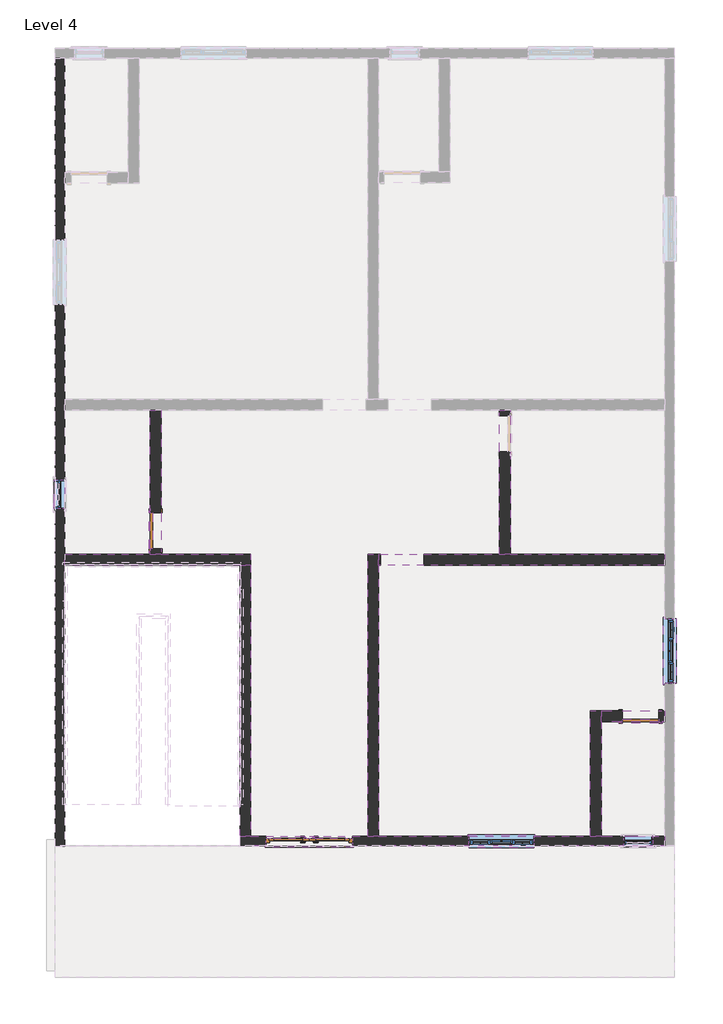
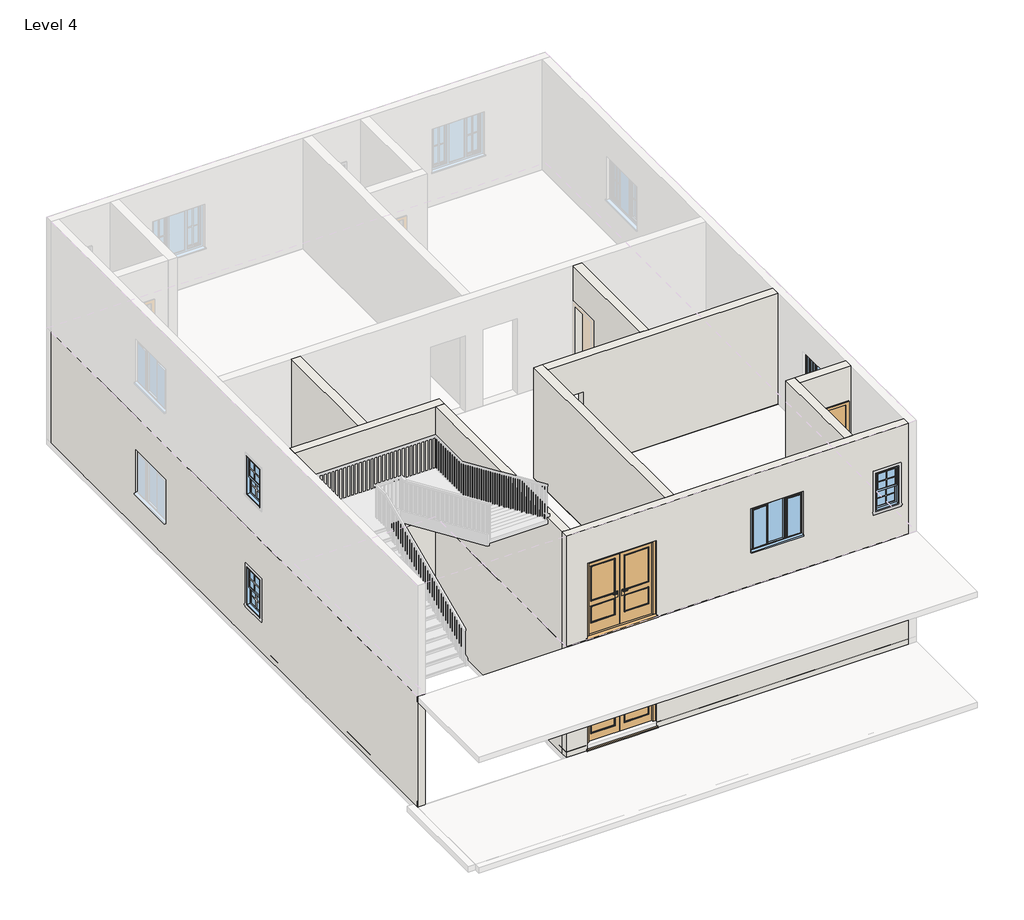
# One storey, part 1 of 5: 29 walls, 12 windows, 9 doors.
"""IFC4 building model written with IfcOpenShell, lengths in millimetres."""

from ifc_helpers import new_model, si_unit, frame, origin, place, context, project, spatial, polyline, outline, extrude, faceted_brep, transform, mapped, element, save
from components import doors_extdbl_2_1810x2110mm_9ab1935a, doors_extdbl_2_1810x2110mm_b7024f51, door_85036156, window_679d2811, windows_tpl_w_glazing_cross_bars_1360x1210mm_0306471f

model = new_model("IFC4")

# Units and contexts
model_context = context("Model", 3, world=origin())
ifc_project = project(units=[si_unit("LENGTHUNIT", "METRE", prefix="MILLI")], contexts=[model_context])

# Site, building, storey
site = spatial("IfcSite", under=ifc_project)
building = spatial("IfcBuilding", under=site)
storey = spatial("IfcBuildingStorey", under=building, Name="Level 4", Elevation=9144.0)

# Doors
placement = place(None, origin())
doors_extdbl_2_1810x2110mm_shape = doors_extdbl_2_1810x2110mm_9ab1935a(model_context)
doors_extdbl_2_1810x2110mm_2_shape = doors_extdbl_2_1810x2110mm_b7024f51(model_context)
element("IfcDoor", 1, ObjectType="Doors_ExtDbl_2 : 1810x2110mm", at=placement, inside=storey, context=model_context, shape_type="MappedRepresentation", body=[
    mapped(doors_extdbl_2_1810x2110mm_shape, transform((-2421.0852725, -7729.5064015, 9144.0), x_axis=(1.0, 0.0, 0.0), y_axis=(0.0, 1.0, 0.0), z_axis=(0.0, 0.0, 1.0))),
    mapped(doors_extdbl_2_1810x2110mm_2_shape, transform((-2421.0852725, -7729.5064015, 9144.0), x_axis=(1.0, 0.0, 0.0), y_axis=(0.0, 1.0, 0.0), z_axis=(0.0, 0.0, 1.0))),
])
element("IfcDoor", 2, ObjectType="Doors_ExtDbl_2 : 1810x2110mm", at=placement, inside=storey, context=model_context, shape_type="MappedRepresentation", body=[
    mapped(doors_extdbl_2_1810x2110mm_shape, transform((-2421.0852725, -7729.5064015, 9144.0), x_axis=(1.0, 0.0, 0.0), y_axis=(0.0, 1.0, 0.0), z_axis=(0.0, 0.0, 1.0))),
    mapped(doors_extdbl_2_1810x2110mm_2_shape, transform((-2421.0852725, -7729.5064015, 9144.0), x_axis=(1.0, 0.0, 0.0), y_axis=(0.0, 1.0, 0.0), z_axis=(0.0, 0.0, 1.0))),
])
element("IfcDoor", 3, ObjectType="Doors_ExtDbl_2 : 1810x2110mm", at=placement, inside=storey, context=model_context, shape_type="MappedRepresentation", body=[
    mapped(doors_extdbl_2_1810x2110mm_shape, transform((-2421.0852725, -7729.5064015, 12192.0), x_axis=(1.0, 0.0, 0.0), y_axis=(0.0, 1.0, 0.0), z_axis=(0.0, 0.0, 1.0))),
    mapped(doors_extdbl_2_1810x2110mm_2_shape, transform((-2421.0852725, -7729.5064015, 12192.0), x_axis=(1.0, 0.0, 0.0), y_axis=(0.0, 1.0, 0.0), z_axis=(0.0, 0.0, 1.0))),
])
door_shape = door_85036156(model_context)
element("IfcDoor", 4, ObjectType="Single-Flush : 30\" x 80\"", at=placement, inside=storey, context=model_context, shape_type="MappedRepresentation", body=[
    mapped(door_shape, transform((-5649.4415084, -1217.2217109, 9144.0), x_axis=(0.0, -1.0, 0.0), y_axis=(1.0, 0.0, 0.0), z_axis=(0.0, 0.0, 1.0))),
])
element("IfcDoor", 5, ObjectType="Single-Flush : 30\" x 80\"", at=placement, inside=storey, context=model_context, shape_type="MappedRepresentation", body=[
    mapped(door_shape, transform((4535.9584916, -5113.3064015, 9144.0), x_axis=(1.0, 0.0, 0.0), y_axis=(0.0, 1.0, 0.0), z_axis=(0.0, 0.0, 1.0))),
])
element("IfcDoor", 6, ObjectType="Single-Flush : 30\" x 80\"", at=placement, inside=storey, context=model_context, shape_type="MappedRepresentation", body=[
    mapped(door_shape, transform((-5649.4415084, -1217.2217109, 9144.0), x_axis=(0.0, -1.0, 0.0), y_axis=(1.0, 0.0, 0.0), z_axis=(0.0, 0.0, 1.0))),
])
element("IfcDoor", 7, ObjectType="Single-Flush : 30\" x 80\"", at=placement, inside=storey, context=model_context, shape_type="MappedRepresentation", body=[
    mapped(door_shape, transform((4535.9584916, -5113.3064015, 9144.0), x_axis=(1.0, 0.0, 0.0), y_axis=(0.0, 1.0, 0.0), z_axis=(0.0, 0.0, 1.0))),
])
element("IfcDoor", 8, ObjectType="Single-Flush : 30\" x 80\"", at=placement, inside=storey, context=model_context, shape_type="MappedRepresentation", body=[
    mapped(door_shape, transform((-5649.4415084, -1217.2217109, 12192.0), x_axis=(0.0, -1.0, 0.0), y_axis=(1.0, 0.0, 0.0), z_axis=(0.0, 0.0, 1.0))),
])
element("IfcDoor", 9, ObjectType="Single-Flush : 30\" x 80\"", at=placement, inside=storey, context=model_context, shape_type="MappedRepresentation", body=[
    mapped(door_shape, transform((4535.9584916, -5113.3064015, 12192.0), x_axis=(1.0, 0.0, 0.0), y_axis=(0.0, 1.0, 0.0), z_axis=(0.0, 0.0, 1.0))),
])

# Walls
element("IfcWall", 10, ObjectType="Generic - 4.5\"", at=placement, inside=storey, context=model_context, shape_type="SweptSolid", body=[
    extrude(outline(polyline([(-1598.2217109, 11176.0), (-1598.2217109, 9144.0), (-1712.5217109, 9144.0), (-1712.5217109, 12192.0), (1312.8935985, 12192.0), (1312.8935985, 9144.0), (-836.2217109, 9144.0), (-836.2217109, 11176.0), (-1598.2217109, 11176.0)])), frame((-5763.7415084, 0.0, 0.0), z_axis=(1.0, 0.0, 0.0), x_axis=(0.0, 1.0, 0.0)), (0.0, 0.0, 1.0), 228.6),
])
element("IfcWall", 11, ObjectType="Generic - 4.5\"", at=placement, inside=storey, context=model_context, shape_type="Brep", body=[
    faceted_brep([(-7554.4415084, -1941.1217109, 9144.0), (-3879.0290366, -1941.1217109, 9144.0), (-3650.4290366, -1941.1217109, 9144.0), (-3650.4290366, -1941.1217109, 12192.0), (-3879.0290366, -1941.1217109, 12192.0), (-7554.4415084, -1941.1217109, 12192.0), (-7554.4415084, -1712.5217109, 9144.0), (-7554.4415084, -1712.5217109, 12192.0), (-5763.7415084, -1712.5217109, 12192.0), (-5535.1415084, -1712.5217109, 12192.0), (-3650.4290366, -1712.5217109, 12192.0), (-3650.4290366, -1712.5217109, 9144.0), (-5535.1415084, -1712.5217109, 9144.0), (-5763.7415084, -1712.5217109, 9144.0)], [[[0, 1, 2, 3, 4, 5]], [[6, 7, 8, 9, 10, 11, 12, 13]], [[2, 1, 0, 6, 13, 12, 11]], [[5, 4, 3, 10, 9, 8, 7]], [[0, 5, 7, 6]], [[3, 2, 11, 10]]]),
])
element("IfcWall", 12, ObjectType="Generic - 4.5\"", at=placement, inside=storey, context=model_context, shape_type="SweptSolid", body=[
    extrude(outline(polyline([(-3879.0290366, -7627.9064015), (-3879.0290366, -1941.1217109), (-3650.4290366, -1941.1217109), (-3650.4290366, -7627.9064015), (-3879.0290366, -7627.9064015)])), frame((0.0, 0.0, 9144.0), z_axis=(0.0, 0.0, 1.0), x_axis=(1.0, 0.0, 0.0)), (0.0, 0.0, 1.0), 3048.0),
])
element("IfcWall", 13, ObjectType="Generic - 4.5\"", at=placement, inside=storey, context=model_context, shape_type="SweptSolid", body=[
    extrude(outline(polyline([(1312.8935985, 9144.0), (1198.5935985, 9144.0), (1198.5935985, 11176.0), (436.5935985, 11176.0), (436.5935985, 9144.0), (-1712.5217109, 9144.0), (-1712.5217109, 12192.0), (1312.8935985, 12192.0), (1312.8935985, 9144.0)])), frame((1576.8584916, 0.0, 0.0), z_axis=(1.0, 0.0, 0.0), x_axis=(0.0, 1.0, 0.0)), (0.0, 0.0, 1.0), 228.6),
])
element("IfcWall", 14, ObjectType="Generic - 4.5\"", at=placement, inside=storey, context=model_context, shape_type="Brep", body=[
    faceted_brep([(-963.1415084, -7627.9064015, 9144.0), (-963.1415084, -1941.1217109, 9144.0), (-963.1415084, -1712.5217109, 9144.0), (-963.1415084, -1712.5217109, 12192.0), (-963.1415084, -1941.1217109, 12192.0), (-963.1415084, -7627.9064015, 12192.0), (-1191.7415084, -7627.9064015, 9144.0), (-1191.7415084, -7627.9064015, 12192.0), (-1191.7415084, -1712.5217109, 12192.0), (-1191.7415084, -1712.5217109, 9144.0)], [[[0, 1, 2, 3, 4, 5]], [[6, 7, 8, 9]], [[2, 1, 0, 6, 9]], [[5, 4, 3, 8, 7]], [[0, 5, 7, 6]], [[3, 2, 9, 8]]]),
])
element("IfcWall", 15, ObjectType="Generic - 4.5\"", at=placement, inside=storey, context=model_context, shape_type="Brep", body=[
    faceted_brep([(-922.8415084, -1712.5217109, 11254.0), (-922.8415084, -1712.5217109, 9144.0), (-963.1415084, -1712.5217109, 9144.0), (-963.1415084, -1712.5217109, 12192.0), (1576.8584916, -1712.5217109, 12192.0), (1805.4584916, -1712.5217109, 12192.0), (5043.9584916, -1712.5217109, 12192.0), (5043.9584916, -1712.5217109, 9144.0), (1805.4584916, -1712.5217109, 9144.0), (1576.8584916, -1712.5217109, 9144.0), (-12.8415084, -1712.5217109, 9144.0), (-12.8415084, -1712.5217109, 11254.0), (-963.1415084, -1941.1217109, 9144.0), (-922.8415084, -1941.1217109, 9144.0), (-922.8415084, -1941.1217109, 11254.0), (-12.8415084, -1941.1217109, 11254.0), (-12.8415084, -1941.1217109, 9144.0), (5043.9584916, -1941.1217109, 9144.0), (5043.9584916, -1941.1217109, 12192.0), (-963.1415084, -1941.1217109, 12192.0)], [[[0, 1, 2, 3, 4, 5, 6, 7, 8, 9, 10, 11]], [[12, 13, 14, 15, 16, 17, 18, 19]], [[2, 1, 13, 12]], [[10, 9, 8, 7, 17, 16]], [[6, 5, 4, 3, 19, 18]], [[3, 2, 12, 19]], [[7, 6, 18, 17]], [[16, 15, 11, 10]], [[14, 13, 1, 0]], [[15, 14, 0, 11]]]),
])
element("IfcWall", 16, ObjectType="Generic - 4.5\"", at=placement, inside=storey, context=model_context, shape_type="Brep", body=[
    faceted_brep([(3710.4584916, -7627.9064015, 9144.0), (3710.4584916, -5227.6064015, 9144.0), (3710.4584916, -4999.0064015, 9144.0), (3710.4584916, -4999.0064015, 12192.0), (3710.4584916, -5227.6064015, 12192.0), (3710.4584916, -7627.9064015, 12192.0), (3481.8584916, -7627.9064015, 9144.0), (3481.8584916, -7627.9064015, 12192.0), (3481.8584916, -4999.0064015, 12192.0), (3481.8584916, -4999.0064015, 9144.0)], [[[0, 1, 2, 3, 4, 5]], [[6, 7, 8, 9]], [[2, 1, 0, 6, 9]], [[5, 4, 3, 8, 7]], [[0, 5, 7, 6]], [[3, 2, 9, 8]]]),
])
element("IfcWall", 17, ObjectType="Generic - 4.5\"", at=placement, inside=storey, context=model_context, shape_type="SweptSolid", body=[
    extrude(outline(polyline([(11176.0, 4916.9584916), (9144.0, 4916.9584916), (9144.0, 5043.9584916), (12192.0, 5043.9584916), (12192.0, 3710.4584916), (9144.0, 3710.4584916), (9144.0, 4154.9584916), (11176.0, 4154.9584916), (11176.0, 4916.9584916)])), frame((0.0, -5227.6064015, 0.0), z_axis=(0.0, 1.0, 0.0), x_axis=(0.0, 0.0, 1.0)), (0.0, 0.0, 1.0), 228.6),
])
element("IfcWall", 18, ObjectType="Generic - 4.5\"", at=placement, inside=storey, context=model_context, shape_type="SweptSolid", body=[
    extrude(outline(polyline([(-1598.2217109, 11176.0), (-1598.2217109, 9144.0), (-1712.5217109, 9144.0), (-1712.5217109, 12192.0), (1312.8935985, 12192.0), (1312.8935985, 9144.0), (-836.2217109, 9144.0), (-836.2217109, 11176.0), (-1598.2217109, 11176.0)])), frame((-5763.7415084, 0.0, 0.0), z_axis=(1.0, 0.0, 0.0), x_axis=(0.0, 1.0, 0.0)), (0.0, 0.0, 1.0), 228.6),
])
element("IfcWall", 19, ObjectType="Generic - 4.5\"", at=placement, inside=storey, context=model_context, shape_type="Brep", body=[
    faceted_brep([(-7554.4415084, -1941.1217109, 9144.0), (-3879.0290366, -1941.1217109, 9144.0), (-3879.0290366, -1941.1217109, 12192.0), (-7554.4415084, -1941.1217109, 12192.0), (-7554.4415084, -1712.5217109, 9144.0), (-7554.4415084, -1712.5217109, 12192.0), (-5763.7415084, -1712.5217109, 12192.0), (-5535.1415084, -1712.5217109, 12192.0), (-3879.0290366, -1712.5217109, 12192.0), (-3879.0290366, -1712.5217109, 9144.0), (-5535.1415084, -1712.5217109, 9144.0), (-5763.7415084, -1712.5217109, 9144.0)], [[[0, 1, 2, 3]], [[4, 5, 6, 7, 8, 9, 10, 11]], [[1, 0, 4, 11, 10, 9]], [[3, 2, 8, 7, 6, 5]], [[0, 3, 5, 4]], [[2, 1, 9, 8]]]),
])
element("IfcWall", 20, ObjectType="Generic - 4.5\"", at=placement, inside=storey, context=model_context, shape_type="SweptSolid", body=[
    extrude(outline(polyline([(-3879.0290366, -7627.9064015), (-3879.0290366, -1941.1217109), (-3650.4290366, -1941.1217109), (-3650.4290366, -7627.9064015), (-3879.0290366, -7627.9064015)])), frame((0.0, 0.0, 9144.0), z_axis=(0.0, 0.0, 1.0), x_axis=(1.0, 0.0, 0.0)), (0.0, 0.0, 1.0), 3048.0),
])
element("IfcWall", 21, ObjectType="Generic - 4.5\"", at=placement, inside=storey, context=model_context, shape_type="SweptSolid", body=[
    extrude(outline(polyline([(1312.8935985, 9144.0), (1198.5935985, 9144.0), (1198.5935985, 11176.0), (436.5935985, 11176.0), (436.5935985, 9144.0), (-1712.5217109, 9144.0), (-1712.5217109, 12192.0), (1312.8935985, 12192.0), (1312.8935985, 9144.0)])), frame((1576.8584916, 0.0, 0.0), z_axis=(1.0, 0.0, 0.0), x_axis=(0.0, 1.0, 0.0)), (0.0, 0.0, 1.0), 228.6),
])
element("IfcWall", 22, ObjectType="Generic - 4.5\"", at=placement, inside=storey, context=model_context, shape_type="SweptSolid", body=[
    extrude(outline(polyline([(-963.1415084, -1941.1217109), (-963.1415084, -7627.9064015), (-1191.7415084, -7627.9064015), (-1191.7415084, -1941.1217109), (-963.1415084, -1941.1217109)])), frame((0.0, 0.0, 9144.0), z_axis=(0.0, 0.0, 1.0), x_axis=(1.0, 0.0, 0.0)), (0.0, 0.0, 1.0), 3048.0),
])
element("IfcWall", 23, ObjectType="Generic - 4.5\"", at=placement, inside=storey, context=model_context, shape_type="Brep", body=[
    faceted_brep([(-922.8415084, -1712.5217109, 11254.0), (-922.8415084, -1712.5217109, 9144.0), (-963.1415084, -1712.5217109, 9144.0), (-963.1415084, -1712.5217109, 12192.0), (1576.8584916, -1712.5217109, 12192.0), (1805.4584916, -1712.5217109, 12192.0), (5043.9584916, -1712.5217109, 12192.0), (5043.9584916, -1712.5217109, 9144.0), (1805.4584916, -1712.5217109, 9144.0), (1576.8584916, -1712.5217109, 9144.0), (-12.8415084, -1712.5217109, 9144.0), (-12.8415084, -1712.5217109, 11254.0), (-963.1415084, -1941.1217109, 9144.0), (-922.8415084, -1941.1217109, 9144.0), (-922.8415084, -1941.1217109, 11254.0), (-12.8415084, -1941.1217109, 11254.0), (-12.8415084, -1941.1217109, 9144.0), (5043.9584916, -1941.1217109, 9144.0), (5043.9584916, -1941.1217109, 12192.0), (-963.1415084, -1941.1217109, 12192.0)], [[[0, 1, 2, 3, 4, 5, 6, 7, 8, 9, 10, 11]], [[12, 13, 14, 15, 16, 17, 18, 19]], [[2, 1, 13, 12]], [[10, 9, 8, 7, 17, 16]], [[6, 5, 4, 3, 19, 18]], [[7, 6, 18, 17]], [[16, 15, 11, 10]], [[14, 13, 1, 0]], [[15, 14, 0, 11]], [[3, 2, 12, 19]]]),
])
element("IfcWall", 24, ObjectType="Generic - 4.5\"", at=placement, inside=storey, context=model_context, shape_type="SweptSolid", body=[
    extrude(outline(polyline([(3710.4584916, -5227.6064015), (3710.4584916, -7627.9064015), (3481.8584916, -7627.9064015), (3481.8584916, -5227.6064015), (3710.4584916, -5227.6064015)])), frame((0.0, 0.0, 9144.0), z_axis=(0.0, 0.0, 1.0), x_axis=(1.0, 0.0, 0.0)), (0.0, 0.0, 1.0), 3048.0),
])
element("IfcWall", 25, ObjectType="Generic - 4.5\"", at=placement, inside=storey, context=model_context, shape_type="SweptSolid", body=[
    extrude(outline(polyline([(11176.0, 4916.9584916), (9144.0, 4916.9584916), (9144.0, 5043.9584916), (12192.0, 5043.9584916), (12192.0, 3710.4584916), (9144.0, 3710.4584916), (9144.0, 4154.9584916), (11176.0, 4154.9584916), (11176.0, 4916.9584916)])), frame((0.0, -5227.6064015, 0.0), z_axis=(0.0, 1.0, 0.0), x_axis=(0.0, 0.0, 1.0)), (0.0, 0.0, 1.0), 228.6),
])
element("IfcWall", 26, ObjectType="Generic - 4.5\"", at=placement, inside=storey, context=model_context, shape_type="SweptSolid", body=[
    extrude(outline(polyline([(-1598.2217109, 14224.0), (-1598.2217109, 12192.0), (-1712.5217109, 12192.0), (-1712.5217109, 15240.0), (1312.8935985, 15240.0), (1312.8935985, 12192.0), (-836.2217109, 12192.0), (-836.2217109, 14224.0), (-1598.2217109, 14224.0)])), frame((-5763.7415084, 0.0, 0.0), z_axis=(1.0, 0.0, 0.0), x_axis=(0.0, 1.0, 0.0)), (0.0, 0.0, 1.0), 228.6),
])
element("IfcWall", 27, ObjectType="Generic - 4.5\"", at=placement, inside=storey, context=model_context, shape_type="Brep", body=[
    faceted_brep([(-7554.4415084, -1941.1217109, 12192.0), (-3879.0290366, -1941.1217109, 12192.0), (-3650.4290366, -1941.1217109, 12192.0), (-3650.4290366, -1941.1217109, 15240.0), (-3879.0290366, -1941.1217109, 15240.0), (-7554.4415084, -1941.1217109, 15240.0), (-7554.4415084, -1712.5217109, 12192.0), (-7554.4415084, -1712.5217109, 15240.0), (-5763.7415084, -1712.5217109, 15240.0), (-5535.1415084, -1712.5217109, 15240.0), (-3650.4290366, -1712.5217109, 15240.0), (-3650.4290366, -1712.5217109, 12192.0), (-5535.1415084, -1712.5217109, 12192.0), (-5763.7415084, -1712.5217109, 12192.0)], [[[0, 1, 2, 3, 4, 5]], [[6, 7, 8, 9, 10, 11, 12, 13]], [[2, 1, 0, 6, 13, 12, 11]], [[5, 4, 3, 10, 9, 8, 7]], [[0, 5, 7, 6]], [[3, 2, 11, 10]]]),
])
element("IfcWall", 28, ObjectType="Generic - 4.5\"", at=placement, inside=storey, context=model_context, shape_type="SweptSolid", body=[
    extrude(outline(polyline([(-3879.0290366, -7627.9064015), (-3879.0290366, -1941.1217109), (-3650.4290366, -1941.1217109), (-3650.4290366, -7627.9064015), (-3879.0290366, -7627.9064015)])), frame((0.0, 0.0, 12192.0), z_axis=(0.0, 0.0, 1.0), x_axis=(1.0, 0.0, 0.0)), (0.0, 0.0, 1.0), 3048.0),
])
element("IfcWall", 29, ObjectType="Generic - 4.5\"", at=placement, inside=storey, context=model_context, shape_type="SweptSolid", body=[
    extrude(outline(polyline([(1312.8935985, 12192.0), (1198.5935985, 12192.0), (1198.5935985, 14224.0), (436.5935985, 14224.0), (436.5935985, 12192.0), (-1712.5217109, 12192.0), (-1712.5217109, 15240.0), (1312.8935985, 15240.0), (1312.8935985, 12192.0)])), frame((1576.8584916, 0.0, 0.0), z_axis=(1.0, 0.0, 0.0), x_axis=(0.0, 1.0, 0.0)), (0.0, 0.0, 1.0), 228.6),
])
element("IfcWall", 30, ObjectType="Generic - 4.5\"", at=placement, inside=storey, context=model_context, shape_type="Brep", body=[
    faceted_brep([(-963.1415084, -7627.9064015, 12192.0), (-963.1415084, -1941.1217109, 12192.0), (-963.1415084, -1712.5217109, 12192.0), (-963.1415084, -1712.5217109, 15240.0), (-963.1415084, -1941.1217109, 15240.0), (-963.1415084, -7627.9064015, 15240.0), (-1191.7415084, -7627.9064015, 12192.0), (-1191.7415084, -7627.9064015, 15240.0), (-1191.7415084, -1712.5217109, 15240.0), (-1191.7415084, -1712.5217109, 12192.0)], [[[0, 1, 2, 3, 4, 5]], [[6, 7, 8, 9]], [[2, 1, 0, 6, 9]], [[5, 4, 3, 8, 7]], [[0, 5, 7, 6]], [[3, 2, 9, 8]]]),
])
element("IfcWall", 31, ObjectType="Generic - 4.5\"", at=placement, inside=storey, context=model_context, shape_type="Brep", body=[
    faceted_brep([(-922.8415084, -1712.5217109, 14302.0), (-922.8415084, -1712.5217109, 12192.0), (-963.1415084, -1712.5217109, 12192.0), (-963.1415084, -1712.5217109, 15240.0), (1576.8584916, -1712.5217109, 15240.0), (1805.4584916, -1712.5217109, 15240.0), (5043.9584916, -1712.5217109, 15240.0), (5043.9584916, -1712.5217109, 12192.0), (1805.4584916, -1712.5217109, 12192.0), (1576.8584916, -1712.5217109, 12192.0), (-12.8415084, -1712.5217109, 12192.0), (-12.8415084, -1712.5217109, 14302.0), (-963.1415084, -1941.1217109, 12192.0), (-922.8415084, -1941.1217109, 12192.0), (-922.8415084, -1941.1217109, 14302.0), (-12.8415084, -1941.1217109, 14302.0), (-12.8415084, -1941.1217109, 12192.0), (5043.9584916, -1941.1217109, 12192.0), (5043.9584916, -1941.1217109, 15240.0), (-963.1415084, -1941.1217109, 15240.0)], [[[0, 1, 2, 3, 4, 5, 6, 7, 8, 9, 10, 11]], [[12, 13, 14, 15, 16, 17, 18, 19]], [[2, 1, 13, 12]], [[10, 9, 8, 7, 17, 16]], [[6, 5, 4, 3, 19, 18]], [[3, 2, 12, 19]], [[7, 6, 18, 17]], [[16, 15, 11, 10]], [[14, 13, 1, 0]], [[15, 14, 0, 11]]]),
])
element("IfcWall", 32, ObjectType="Generic - 4.5\"", at=placement, inside=storey, context=model_context, shape_type="Brep", body=[
    faceted_brep([(3710.4584916, -7627.9064015, 12192.0), (3710.4584916, -5227.6064015, 12192.0), (3710.4584916, -4999.0064015, 12192.0), (3710.4584916, -4999.0064015, 15240.0), (3710.4584916, -5227.6064015, 15240.0), (3710.4584916, -7627.9064015, 15240.0), (3481.8584916, -7627.9064015, 12192.0), (3481.8584916, -7627.9064015, 15240.0), (3481.8584916, -4999.0064015, 15240.0), (3481.8584916, -4999.0064015, 12192.0)], [[[0, 1, 2, 3, 4, 5]], [[6, 7, 8, 9]], [[2, 1, 0, 6, 9]], [[5, 4, 3, 8, 7]], [[0, 5, 7, 6]], [[3, 2, 9, 8]]]),
])
element("IfcWall", 33, ObjectType="Generic - 4.5\"", at=placement, inside=storey, context=model_context, shape_type="SweptSolid", body=[
    extrude(outline(polyline([(14224.0, 4916.9584916), (12192.0, 4916.9584916), (12192.0, 5043.9584916), (15240.0, 5043.9584916), (15240.0, 3710.4584916), (12192.0, 3710.4584916), (12192.0, 4154.9584916), (14224.0, 4154.9584916), (14224.0, 4916.9584916)])), frame((0.0, -5227.6064015, 0.0), z_axis=(0.0, 1.0, 0.0), x_axis=(0.0, 0.0, 1.0)), (0.0, 0.0, 1.0), 228.6),
])
element("IfcWall", 34, ObjectType="Generic - 9\"", at=placement, inside=storey, context=model_context, shape_type="Brep", body=[
    faceted_brep([(5043.9584916, -7627.9064015, 9144.0), (3710.4584916, -7627.9064015, 9144.0), (3481.8584916, -7627.9064015, 9144.0), (-963.1415084, -7627.9064015, 9144.0), (-1191.7415084, -7627.9064015, 9144.0), (-1516.0852725, -7627.9064015, 9144.0), (-1516.0852725, -7627.9064015, 11254.0), (-3326.0852725, -7627.9064015, 11254.0), (-3326.0852725, -7627.9064015, 9144.0), (-3650.4290366, -7627.9064015, 9144.0), (-3879.0290366, -7627.9064015, 9144.0), (-3879.0290366, -7627.9064015, 12192.0), (-3650.4290366, -7627.9064015, 12192.0), (-1191.7415084, -7627.9064015, 12192.0), (-963.1415084, -7627.9064015, 12192.0), (3481.8584916, -7627.9064015, 12192.0), (3710.4584916, -7627.9064015, 12192.0), (5043.9584916, -7627.9064015, 12192.0), (2294.9584916, -7627.9064015, 11268.4), (934.9584916, -7627.9064015, 11268.4), (934.9584916, -7627.9064015, 10058.4), (2294.9584916, -7627.9064015, 10058.4), (4789.9584916, -7627.9064015, 11125.2), (4180.3584916, -7627.9064015, 11125.2), (4180.3584916, -7627.9064015, 10058.4), (4789.9584916, -7627.9064015, 10058.4), (-1516.0852725, -7831.1064015, 11254.0), (-1516.0852725, -7831.1064015, 9144.0), (5043.9584916, -7831.1064015, 9144.0), (5043.9584916, -7831.1064015, 12192.0), (-3879.0290366, -7831.1064015, 12192.0), (-3879.0290366, -7831.1064015, 9144.0), (-3326.0852725, -7831.1064015, 9144.0), (-3326.0852725, -7831.1064015, 11254.0), (2294.9584916, -7831.1064015, 11268.4), (2294.9584916, -7831.1064015, 10058.4), (934.9584916, -7831.1064015, 10058.4), (934.9584916, -7831.1064015, 11268.4), (4789.9584916, -7831.1064015, 11125.2), (4789.9584916, -7831.1064015, 10058.4), (4180.3584916, -7831.1064015, 10058.4), (4180.3584916, -7831.1064015, 11125.2)], [[[0, 1, 2, 3, 4, 5, 6, 7, 8, 9, 10, 11, 12, 13, 14, 15, 16, 17], [18, 19, 20, 21], [22, 23, 24, 25]], [[26, 27, 28, 29, 30, 31, 32, 33], [34, 35, 36, 37], [38, 39, 40, 41]], [[32, 31, 10, 9, 8]], [[28, 27, 5, 4, 3, 2, 1, 0]], [[17, 16, 15, 14, 13, 12, 11, 30, 29]], [[11, 10, 31, 30]], [[35, 34, 18, 21]], [[36, 35, 21, 20]], [[37, 36, 20, 19]], [[34, 37, 19, 18]], [[39, 38, 22, 25]], [[40, 39, 25, 24]], [[41, 40, 24, 23]], [[38, 41, 23, 22]], [[8, 7, 33, 32]], [[6, 5, 27, 26]], [[7, 6, 26, 33]], [[0, 17, 29, 28]]]),
])
element("IfcWall", 35, ObjectType="Generic - 9\"", at=placement, inside=storey, context=model_context, shape_type="Brep", body=[
    faceted_brep([(-7757.6415084, 8704.2935985, 9144.0), (-7757.6415084, -7843.8064015, 9144.0), (-7757.6415084, -7843.8064015, 12192.0), (-7757.6415084, 8704.2935985, 12192.0), (-7757.6415084, 3528.4935985, 11268.4), (-7757.6415084, 3528.4935985, 10058.4), (-7757.6415084, 4888.4935985, 10058.4), (-7757.6415084, 4888.4935985, 11268.4), (-7757.6415084, -760.0217109, 11125.2), (-7757.6415084, -760.0217109, 10058.4), (-7757.6415084, -150.4217109, 10058.4), (-7757.6415084, -150.4217109, 11125.2), (-7554.4415084, 8704.2935985, 9144.0), (-7554.4415084, 8704.2935985, 12192.0), (-7554.4415084, 6303.9935985, 12192.0), (-7554.4415084, 6075.3935985, 12192.0), (-7554.4415084, 1541.4935985, 12192.0), (-7554.4415084, 1312.8935985, 12192.0), (-7554.4415084, -1712.5217109, 12192.0), (-7554.4415084, -1941.1217109, 12192.0), (-7554.4415084, -7843.8064015, 12192.0), (-7554.4415084, -7843.8064015, 9144.0), (-7554.4415084, -1941.1217109, 9144.0), (-7554.4415084, -1712.5217109, 9144.0), (-7554.4415084, 1312.8935985, 9144.0), (-7554.4415084, 1541.4935985, 9144.0), (-7554.4415084, 6075.3935985, 9144.0), (-7554.4415084, 6303.9935985, 9144.0), (-7554.4415084, 3528.4935985, 11268.4), (-7554.4415084, 4888.4935985, 11268.4), (-7554.4415084, 4888.4935985, 10058.4), (-7554.4415084, 3528.4935985, 10058.4), (-7554.4415084, -760.0217109, 11125.2), (-7554.4415084, -150.4217109, 11125.2), (-7554.4415084, -150.4217109, 10058.4), (-7554.4415084, -760.0217109, 10058.4)], [[[0, 1, 2, 3], [4, 5, 6, 7], [8, 9, 10, 11]], [[12, 13, 14, 15, 16, 17, 18, 19, 20, 21, 22, 23, 24, 25, 26, 27], [28, 29, 30, 31], [32, 33, 34, 35]], [[1, 0, 12, 27, 26, 25, 24, 23, 22, 21]], [[2, 1, 21, 20]], [[3, 2, 20, 19, 18, 17, 16, 15, 14, 13]], [[5, 4, 28, 31]], [[6, 5, 31, 30]], [[7, 6, 30, 29]], [[4, 7, 29, 28]], [[9, 8, 32, 35]], [[10, 9, 35, 34]], [[11, 10, 34, 33]], [[8, 11, 33, 32]], [[0, 3, 13, 12]]]),
])
element("IfcWall", 36, ObjectType="Generic - 9\"", at=placement, inside=storey, context=model_context, shape_type="Brep", body=[
    faceted_brep([(5043.9584916, -7627.9064015, 9144.0), (3710.4584916, -7627.9064015, 9144.0), (3481.8584916, -7627.9064015, 9144.0), (-963.1415084, -7627.9064015, 9144.0), (-1191.7415084, -7627.9064015, 9144.0), (-1516.0852725, -7627.9064015, 9144.0), (-1516.0852725, -7627.9064015, 11254.0), (-3326.0852725, -7627.9064015, 11254.0), (-3326.0852725, -7627.9064015, 9144.0), (-3650.4290366, -7627.9064015, 9144.0), (-3650.4290366, -7627.9064015, 12192.0), (-1191.7415084, -7627.9064015, 12192.0), (-963.1415084, -7627.9064015, 12192.0), (3481.8584916, -7627.9064015, 12192.0), (3710.4584916, -7627.9064015, 12192.0), (5043.9584916, -7627.9064015, 12192.0), (2294.9584916, -7627.9064015, 11268.4), (934.9584916, -7627.9064015, 11268.4), (934.9584916, -7627.9064015, 10058.4), (2294.9584916, -7627.9064015, 10058.4), (4789.9584916, -7627.9064015, 11125.2), (4180.3584916, -7627.9064015, 11125.2), (4180.3584916, -7627.9064015, 10058.4), (4789.9584916, -7627.9064015, 10058.4), (-1516.0852725, -7831.1064015, 11254.0), (-1516.0852725, -7831.1064015, 9144.0), (5043.9584916, -7831.1064015, 9144.0), (5043.9584916, -7831.1064015, 12192.0), (-3650.4290366, -7831.1064015, 12192.0), (-3650.4290366, -7831.1064015, 9144.0), (-3326.0852725, -7831.1064015, 9144.0), (-3326.0852725, -7831.1064015, 11254.0), (2294.9584916, -7831.1064015, 11268.4), (2294.9584916, -7831.1064015, 10058.4), (934.9584916, -7831.1064015, 10058.4), (934.9584916, -7831.1064015, 11268.4), (4789.9584916, -7831.1064015, 11125.2), (4789.9584916, -7831.1064015, 10058.4), (4180.3584916, -7831.1064015, 10058.4), (4180.3584916, -7831.1064015, 11125.2)], [[[0, 1, 2, 3, 4, 5, 6, 7, 8, 9, 10, 11, 12, 13, 14, 15], [16, 17, 18, 19], [20, 21, 22, 23]], [[24, 25, 26, 27, 28, 29, 30, 31], [32, 33, 34, 35], [36, 37, 38, 39]], [[30, 29, 9, 8]], [[26, 25, 5, 4, 3, 2, 1, 0]], [[15, 14, 13, 12, 11, 10, 28, 27]], [[33, 32, 16, 19]], [[34, 33, 19, 18]], [[35, 34, 18, 17]], [[32, 35, 17, 16]], [[37, 36, 20, 23]], [[38, 37, 23, 22]], [[39, 38, 22, 21]], [[36, 39, 21, 20]], [[8, 7, 31, 30]], [[6, 5, 25, 24]], [[7, 6, 24, 31]], [[10, 9, 29, 28]], [[0, 15, 27, 26]]]),
])
element("IfcWall", 37, ObjectType="Generic - 9\"", at=placement, inside=storey, context=model_context, shape_type="Brep", body=[
    faceted_brep([(-7757.6415084, 8704.2935985, 9144.0), (-7757.6415084, -7843.8064015, 9144.0), (-7757.6415084, -7843.8064015, 12192.0), (-7757.6415084, 8704.2935985, 12192.0), (-7757.6415084, 3528.4935985, 11268.4), (-7757.6415084, 3528.4935985, 10058.4), (-7757.6415084, 4888.4935985, 10058.4), (-7757.6415084, 4888.4935985, 11268.4), (-7757.6415084, -760.0217109, 11125.2), (-7757.6415084, -760.0217109, 10058.4), (-7757.6415084, -150.4217109, 10058.4), (-7757.6415084, -150.4217109, 11125.2), (-7554.4415084, 8704.2935985, 9144.0), (-7554.4415084, 8704.2935985, 12192.0), (-7554.4415084, 6303.9935985, 12192.0), (-7554.4415084, 6075.3935985, 12192.0), (-7554.4415084, 1541.4935985, 12192.0), (-7554.4415084, 1312.8935985, 12192.0), (-7554.4415084, -1712.5217109, 12192.0), (-7554.4415084, -1941.1217109, 12192.0), (-7554.4415084, -7843.8064015, 12192.0), (-7554.4415084, -7843.8064015, 9144.0), (-7554.4415084, -1941.1217109, 9144.0), (-7554.4415084, -1712.5217109, 9144.0), (-7554.4415084, 1312.8935985, 9144.0), (-7554.4415084, 1541.4935985, 9144.0), (-7554.4415084, 6075.3935985, 9144.0), (-7554.4415084, 6303.9935985, 9144.0), (-7554.4415084, 3528.4935985, 11268.4), (-7554.4415084, 4888.4935985, 11268.4), (-7554.4415084, 4888.4935985, 10058.4), (-7554.4415084, 3528.4935985, 10058.4), (-7554.4415084, -760.0217109, 11125.2), (-7554.4415084, -150.4217109, 11125.2), (-7554.4415084, -150.4217109, 10058.4), (-7554.4415084, -760.0217109, 10058.4)], [[[0, 1, 2, 3], [4, 5, 6, 7], [8, 9, 10, 11]], [[12, 13, 14, 15, 16, 17, 18, 19, 20, 21, 22, 23, 24, 25, 26, 27], [28, 29, 30, 31], [32, 33, 34, 35]], [[1, 0, 12, 27, 26, 25, 24, 23, 22, 21]], [[2, 1, 21, 20]], [[3, 2, 20, 19, 18, 17, 16, 15, 14, 13]], [[5, 4, 28, 31]], [[6, 5, 31, 30]], [[7, 6, 30, 29]], [[4, 7, 29, 28]], [[9, 8, 32, 35]], [[10, 9, 35, 34]], [[11, 10, 34, 33]], [[8, 11, 33, 32]], [[0, 3, 13, 12]]]),
])
element("IfcWall", 38, ObjectType="Generic - 9\"", at=placement, inside=storey, context=model_context, shape_type="Brep", body=[
    faceted_brep([(5043.9584916, -7627.9064015, 12192.0), (3710.4584916, -7627.9064015, 12192.0), (3481.8584916, -7627.9064015, 12192.0), (-963.1415084, -7627.9064015, 12192.0), (-1191.7415084, -7627.9064015, 12192.0), (-1516.0852725, -7627.9064015, 12192.0), (-1516.0852725, -7627.9064015, 14302.0), (-3326.0852725, -7627.9064015, 14302.0), (-3326.0852725, -7627.9064015, 12192.0), (-3650.4290366, -7627.9064015, 12192.0), (-3879.0290366, -7627.9064015, 12192.0), (-3879.0290366, -7627.9064015, 15240.0), (-3650.4290366, -7627.9064015, 15240.0), (-1191.7415084, -7627.9064015, 15240.0), (-963.1415084, -7627.9064015, 15240.0), (3481.8584916, -7627.9064015, 15240.0), (3710.4584916, -7627.9064015, 15240.0), (5043.9584916, -7627.9064015, 15240.0), (2294.9584916, -7627.9064015, 14316.4), (934.9584916, -7627.9064015, 14316.4), (934.9584916, -7627.9064015, 13106.4), (2294.9584916, -7627.9064015, 13106.4), (4789.9584916, -7627.9064015, 14173.2), (4180.3584916, -7627.9064015, 14173.2), (4180.3584916, -7627.9064015, 13106.4), (4789.9584916, -7627.9064015, 13106.4), (-1516.0852725, -7831.1064015, 14302.0), (-1516.0852725, -7831.1064015, 12192.0), (5043.9584916, -7831.1064015, 12192.0), (5043.9584916, -7831.1064015, 15240.0), (-3879.0290366, -7831.1064015, 15240.0), (-3879.0290366, -7831.1064015, 12192.0), (-3326.0852725, -7831.1064015, 12192.0), (-3326.0852725, -7831.1064015, 14302.0), (2294.9584916, -7831.1064015, 14316.4), (2294.9584916, -7831.1064015, 13106.4), (934.9584916, -7831.1064015, 13106.4), (934.9584916, -7831.1064015, 14316.4), (4789.9584916, -7831.1064015, 14173.2), (4789.9584916, -7831.1064015, 13106.4), (4180.3584916, -7831.1064015, 13106.4), (4180.3584916, -7831.1064015, 14173.2)], [[[0, 1, 2, 3, 4, 5, 6, 7, 8, 9, 10, 11, 12, 13, 14, 15, 16, 17], [18, 19, 20, 21], [22, 23, 24, 25]], [[26, 27, 28, 29, 30, 31, 32, 33], [34, 35, 36, 37], [38, 39, 40, 41]], [[32, 31, 10, 9, 8]], [[28, 27, 5, 4, 3, 2, 1, 0]], [[17, 16, 15, 14, 13, 12, 11, 30, 29]], [[11, 10, 31, 30]], [[35, 34, 18, 21]], [[36, 35, 21, 20]], [[37, 36, 20, 19]], [[34, 37, 19, 18]], [[39, 38, 22, 25]], [[40, 39, 25, 24]], [[41, 40, 24, 23]], [[38, 41, 23, 22]], [[8, 7, 33, 32]], [[6, 5, 27, 26]], [[7, 6, 26, 33]], [[0, 17, 29, 28]]]),
])

# Windows
window_shape = window_679d2811(model_context)
element("IfcWindow", 39, ObjectType="Window-Double-Hung : 24\" x 42\"", at=placement, inside=storey, context=model_context, shape_type="MappedRepresentation", body=[
    mapped(window_shape, transform((-7656.0415084, -455.2217109, 9144.0), x_axis=(0.0, 1.0, 0.0), y_axis=(-1.0, 0.0, 0.0), z_axis=(0.0, 0.0, 1.0))),
])
element("IfcWindow", 40, ObjectType="Window-Double-Hung : 24\" x 42\"", at=placement, inside=storey, context=model_context, shape_type="MappedRepresentation", body=[
    mapped(window_shape, transform((4485.1584916, -7729.5064015, 9144.0), x_axis=(-1.0, 0.0, 0.0), y_axis=(0.0, -1.0, 0.0), z_axis=(0.0, 0.0, 1.0))),
])
element("IfcWindow", 41, ObjectType="Window-Double-Hung : 24\" x 42\"", at=placement, inside=storey, context=model_context, shape_type="MappedRepresentation", body=[
    mapped(window_shape, transform((-7656.0415084, -455.2217109, 9144.0), x_axis=(0.0, 1.0, 0.0), y_axis=(-1.0, 0.0, 0.0), z_axis=(0.0, 0.0, 1.0))),
])
element("IfcWindow", 42, ObjectType="Window-Double-Hung : 24\" x 42\"", at=placement, inside=storey, context=model_context, shape_type="MappedRepresentation", body=[
    mapped(window_shape, transform((4485.1584916, -7729.5064015, 9144.0), x_axis=(-1.0, 0.0, 0.0), y_axis=(0.0, -1.0, 0.0), z_axis=(0.0, 0.0, 1.0))),
])
element("IfcWindow", 43, ObjectType="Window-Double-Hung : 24\" x 42\"", at=placement, inside=storey, context=model_context, shape_type="MappedRepresentation", body=[
    mapped(window_shape, transform((-7656.0415084, -455.2217109, 12192.0), x_axis=(0.0, 1.0, 0.0), y_axis=(-1.0, 0.0, 0.0), z_axis=(0.0, 0.0, 1.0))),
])
element("IfcWindow", 44, ObjectType="Window-Double-Hung : 24\" x 42\"", at=placement, inside=storey, context=model_context, shape_type="MappedRepresentation", body=[
    mapped(window_shape, transform((4485.1584916, -7729.5064015, 12192.0), x_axis=(-1.0, 0.0, 0.0), y_axis=(0.0, -1.0, 0.0), z_axis=(0.0, 0.0, 1.0))),
])
windows_tpl_w_glazing_cross_bars_1360x1210mm_shape = windows_tpl_w_glazing_cross_bars_1360x1210mm_0306471f(model_context)
element("IfcWindow", 45, ObjectType="Windows_Tpl_w-Glazing_Cross-Bars : 1360x1210mm", at=placement, inside=storey, context=model_context, shape_type="MappedRepresentation", body=[
    mapped(windows_tpl_w_glazing_cross_bars_1360x1210mm_shape, transform((5137.1019238, -4243.3730682, 9158.4), x_axis=(0.0, -1.0, 0.0), y_axis=(1.0, 0.0, 0.0), z_axis=(0.0, 0.0, 1.0))),
])
element("IfcWindow", 46, ObjectType="Windows_Tpl_w-Glazing_Cross-Bars : 1360x1210mm", at=placement, inside=storey, context=model_context, shape_type="MappedRepresentation", body=[
    mapped(windows_tpl_w_glazing_cross_bars_1360x1210mm_shape, transform((1113.2918249, -7721.0498337, 9158.4), x_axis=(-1.0, 0.0, 0.0), y_axis=(0.0, -1.0, 0.0), z_axis=(0.0, 0.0, 1.0))),
])
element("IfcWindow", 47, ObjectType="Windows_Tpl_w-Glazing_Cross-Bars : 1360x1210mm", at=placement, inside=storey, context=model_context, shape_type="MappedRepresentation", body=[
    mapped(windows_tpl_w_glazing_cross_bars_1360x1210mm_shape, transform((5137.1019238, -4243.3730682, 9158.4), x_axis=(0.0, -1.0, 0.0), y_axis=(1.0, 0.0, 0.0), z_axis=(0.0, 0.0, 1.0))),
])
element("IfcWindow", 48, ObjectType="Windows_Tpl_w-Glazing_Cross-Bars : 1360x1210mm", at=placement, inside=storey, context=model_context, shape_type="MappedRepresentation", body=[
    mapped(windows_tpl_w_glazing_cross_bars_1360x1210mm_shape, transform((1113.2918249, -7721.0498337, 9158.4), x_axis=(-1.0, 0.0, 0.0), y_axis=(0.0, -1.0, 0.0), z_axis=(0.0, 0.0, 1.0))),
])
element("IfcWindow", 49, ObjectType="Windows_Tpl_w-Glazing_Cross-Bars : 1360x1210mm", at=placement, inside=storey, context=model_context, shape_type="MappedRepresentation", body=[
    mapped(windows_tpl_w_glazing_cross_bars_1360x1210mm_shape, transform((5137.1019238, -4243.3730682, 12206.4), x_axis=(0.0, -1.0, 0.0), y_axis=(1.0, 0.0, 0.0), z_axis=(0.0, 0.0, 1.0))),
])
element("IfcWindow", 50, ObjectType="Windows_Tpl_w-Glazing_Cross-Bars : 1360x1210mm", at=placement, inside=storey, context=model_context, shape_type="MappedRepresentation", body=[
    mapped(windows_tpl_w_glazing_cross_bars_1360x1210mm_shape, transform((1113.2918249, -7721.0498337, 12206.4), x_axis=(-1.0, 0.0, 0.0), y_axis=(0.0, -1.0, 0.0), z_axis=(0.0, 0.0, 1.0))),
])

save(model, "model.ifc")

# Revit data of these elements
# Type "Doors_ExtDbl_2 : 1810x2110mm"
#   Type Mark = "8"
#   Type Comments = "External Double"
#   Operation = "DoubleDoorSingleSwing"
#   Construction Type Id = "GSP4R"
#   Keynote = "L20"
#   Analytic Construction = "1/8 in Pilkington single glazing"
#   Wrap Layers (Int) from Ext = 0' - 6.98819"
#   Wrap Layers (Ext) from Ext = 0' - 4.03543"
#   Visual Light Transmittance = 0.9
#   Top of Lock Rail = 2' - 11.43307"
#   Thickness = 0' - 1.73228"
#   Stile Shutting = 0' - 4.92126"
#   Stile - Top Rail = 0' - 5.90551"
#   Stile - Lock Rail = 0' - 5.90551"
#   Stile - Hanging = 0' - 3.93701"
#   Stile - Bottom Rail = 0' - 11.81102"
#   Solar Heat Gain Coefficient = 0.78
#   Rough Width = 5' - 11.25984"
#   Rough Height = 6' - 11.07087"
#   O/A Frame Width = 0' - 2.51969"
#   Heat Transfer Coefficient (U) = 0.6496 BTU/(h·ft²·°F)
#   Handle Z Distance = 3' - 1.40157"
#   Glazing Thickness = 0' - 0.94488"
#   FrameWidth = 0' - 1.65354"
#   FrameOffset - External = 0' - 2.55906"
#   FrameDepth = 0' - 3.50394"
#   Door Panel Width = 2' - 9.54331"
#   Door Panel Thickness = 0' - 1.73228"
#   Door Panel Height = 6' - 6.74016"
#   Cill Thickness = 0' - 2.14567"
#   Cill Projection = 0' - 1.1811"
#   Handle X Distance = 0' - 2.95276"
#   Height = 6' - 11.07087"
#   Structural Tolerance = 0' - 0.25591"
#   Tolerance = 0' - 0.11811"
#   Undercut = 0' - 0.15748"
#   Width = 5' - 11.25984"
#   Cill Extension = 0' - 0.98425"
#   Cavity Closer Width = 0' - 1.9685"
#   Cavity Closer Offset from Ext = 0' - 4.03543"
#   Cavity Closer Depth = 0' - 3.34646"
#   Vis - Ironmongery = yes
#   Vis - Cavity Closers = yes
#   Define Thermal Properties by = 1
#   Function = 1
#   Material Glass = Door - Glazing
#   Handle Style = element 387460
#   Material Door = Door - Panel
#   Material Frame = Door - Frame/Mullion
#   Material Ironmongery = Door - Handle
#   Wall Closure = (empty or 0)
# Type "Single-Flush : 30\" x 80\""
#   Type Mark = "5"
#   Construction Type Id = "MDOOR"
#   Assembly Code = "C1020"
#   Analytic Construction = "Metal"
#   Thickness = 0' - 2"
#   Heat Transfer Coefficient (U) = 0.651978 BTU/(h·ft²·°F)
#   Height = 6' - 8"
#   Trim Projection Ext = 0' - 1"
#   Trim Projection Int = 0' - 1"
#   Trim Width = 0' - 3"
#   Width = 2' - 6"
#   Define Thermal Properties by = 1
#   Define Thermal Properties by = 1
#   Door Material = Door - Panel
#   Frame Material = Door - Frame
#   Visual Light Transmittance = 0
#   Solar Heat Gain Coefficient = 0
#   Function = (empty or 0)
#   Wall Closure = (empty or 0)
# Type "Generic - 4.5\""
#   Assembly Code = "B2010"
#   Layers, outside or top first: 0' - 9" no material (function 1)
# Type "Generic - 9\""
#   Assembly Code = "B2010"
#   Layers, outside or top first: 0' - 8" no material (function 1)
# Type "Window-Double-Hung : 24\" x 42\""
#   Type Mark = "10"
#   Fire Rating = "0.5h"
#   Construction Type Id = "DG-DR"
#   Assembly Code = "B2020100"
#   Analytic Construction = "Double glazing - domestic"
#   Wall Thickness [instance default] = 0' - 6"
#   Window Inset [instance default] = 0' - 0"
#   Visual Light Transmittance = 0.81
#   Thermal Resistance (R) = 1.8146 (h·ft²·°F)/BTU
#   Solar Heat Gain Coefficient = 0.76
#   Muntin Width = 1' - 6"
#   Muntin Height = 1' - 5 1/8"
#   Interior Wall Closure [instance default] = 0' - 1 1/2"
#   Rough Width = 2' - 0 1/2"
#   Rough Height = 3' - 6 1/2"
#   Frame Extension [instance default] = 0' - 1 1/4"
#   Exterior Wall Closure [instance default] = 0' - 0 1/2"
#   Extension Jamb [instance default] = 0' - 1 1/2"
#   Heat Transfer Coefficient (U) = 0.5511 BTU/(h·ft²·°F)
#   Height = 3' - 6"
#   Width = 2' - 0"
#   Define Thermal Properties by = 1
#   Top Muntin Visibility = yes
#   Indicator Visibility [instance default] = yes
#   Extension Jamb Visibility [instance default] = yes
#   Interior Trim Visibility [instance default] = yes
#   Exterior Trim Visibility [instance default] = yes
#   Define Thermal Properties by = 1
#   Bottom Muntin Visibility = yes
#   Muntin Pattern = Muntin Pattern_2x2 : Muntin Pattern_2x2
#   Interior Trim Material = Wood - Stained
#   Interior Trim = Trim-Window-Interior-Flat : Picture Frame
#   Exterior Trim Material = Clad - White
#   Exterior Trim = Trim-Window-Exterior-Flat : with Sill
#   Glass Panel Material = Glass
#   Exterior Frame Material = Clad - White
#   Interior Frame Material = Wood - Stained
#   Wall Closure = (empty or 0)
# Type "Windows_Tpl_w-Glazing_Cross-Bars : 1360x1210mm"
#   Type Mark = "21"
#   Operation = "TriplePanelVertical"
#   Construction Type Id = "GSP4R"
#   Manufacturer = "Revit"
#   Keynote = "L10"
#   Analytic Construction = "1/8 in Pilkington single glazing"
#   Wrap Layers (Ext) from Ext = 0' - 4.03543"
#   Wrap Layers (Int) from Ext = 0' - 6.98819"
#   Window Board Projection = 0' - 0.98425"
#   Window Board Extension = 0' - 0.98425"
#   Visual Light Transmittance = 0.9
#   Solar Heat Gain Coefficient = 0.78
#   Rough Width = 4' - 5.54331"
#   Rough Height = 3' - 11.6378"
#   Height = 3' - 11.6378"
#   Width = 4' - 5.54331"
#   Heat Transfer Coefficient (U) = 0.6496 BTU/(h·ft²·°F)
#   Glazing Thickness = 0' - 0.94488"
#   Glazing Bar Thickness = 0' - 0.7874"
#   FrameOffset - External = 0' - 1.9685"
#   Frame Depth = 0' - 2.55906"
#   Default Head Height = 6' - 11.07087"
#   Cill Depth = 0' - 3.44488"
#   Cavity Closer Width = 0' - 1.9685"
#   Cavity Closer Offset from Ext = 0' - 4.03543"
#   Cavity Closer Depth = 0' - 3.34646"
#   Vis - Glazing Bars = yes
#   Vis - Cavity Closers = yes
#   Define Thermal Properties by = 1
#   Material Trim = Window Frame
#   Material Glazing Bars = Window Frame
#   Material Glass = Glass
#   Material Frame = Window Frame
#   Wall Closure = (empty or 0)
# Elements 1, 2, 3 (IfcDoor, "Doors_ExtDbl_2 : 1810x2110mm")
#   Phase Created = New Construction
#   Materials on its faces: "Door - Panel", "Door - Handle", "Door - Frame/Mullion", "Door - Glazing"
# Elements 4, 5, 6, 7, 8, 9 (IfcDoor, "Single-Flush : 30\" x 80\"")
#   Phase Created = New Construction
#   Materials on its faces: "Door - Frame", "Door - Panel"
# Elements 10, 11, 12, 13, 14, 15, 16, 17, 18, 21, 22, 23, 24, 25 (IfcWall, "Generic - 4.5\"")
#   Top Offset = 10' - 0"
#   Base Offset = 0' - 0"
#   wall height = 10' - 0"
#   Phase Created = New Construction
#   Base Constraint = Level 4
#   Top Constraint = Level 4
#   Materials on its faces: "Default Wall"
# Element 19 (IfcWall, "Generic - 4.5\"")
#   Top Offset = 10' - 0"
#   Base Offset = 0' - 0"
#   wall height = 10' - 0"
#   Phase Created = New Construction
#   Base Constraint = Level 4
#   Top Constraint = Level 4
#   Materials on its faces: "Default Wall", "Concrete, Precast"
# Element 20 (IfcWall, "Generic - 4.5\"")
#   Top Offset = 10' - 0"
#   Base Offset = 0' - 0"
#   wall height = 10' - 0"
#   Phase Created = New Construction
#   Base Constraint = Level 4
#   Top Constraint = Level 4
#   Materials on its faces: "Default Wall", "Bed-white fabric"
# Elements 26, 29, 30, 31, 32, 33 (IfcWall, "Generic - 4.5\"")
#   built-in parameter 1001111 = 10' - 0"
#   Top Offset = 20' - 0"
#   Base Offset = 10' - 0"
#   wall height = 10' - 0"
#   Phase Created = New Construction
#   Base Constraint = Level 4
#   Top Constraint = Level 4
#   Materials on its faces: "Default Wall"
# Element 27 (IfcWall, "Generic - 4.5\"")
#   built-in parameter 1001111 = 10' - 0"
#   Top Offset = 20' - 0"
#   Base Offset = 10' - 0"
#   wall height = 10' - 0"
#   Phase Created = New Construction
#   Base Constraint = Level 4
#   Top Constraint = Level 4
#   Materials on its faces: "Default Wall", "Concrete, Precast"
# Element 28 (IfcWall, "Generic - 4.5\"")
#   built-in parameter 1001111 = 10' - 0"
#   Top Offset = 20' - 0"
#   Base Offset = 10' - 0"
#   wall height = 10' - 0"
#   Phase Created = New Construction
#   Base Constraint = Level 4
#   Top Constraint = Level 4
#   Materials on its faces: "Default Wall", "Bed-white fabric"
# Elements 34, 36 (IfcWall, "Generic - 9\"")
#   Top Offset = 10' - 0"
#   Base Offset = 0' - 0"
#   wall height = 10' - 0"
#   Phase Created = New Construction
#   Base Constraint = Level 4
#   Top Constraint = Level 4
#   Materials on its faces: "Default Wall", "Bed-night tables"
# Element 35 (IfcWall, "Generic - 9\"")
#   Top Offset = 10' - 0"
#   Base Offset = 0' - 0"
#   wall height = 10' - 0"
#   Phase Created = New Construction
#   Base Constraint = Level 4
#   Top Constraint = Level 4
#   Materials on its faces: "Default Wall"
# Element 37 (IfcWall, "Generic - 9\"")
#   Top Offset = 10' - 0"
#   Base Offset = 0' - 0"
#   wall height = 10' - 0"
#   Phase Created = New Construction
#   Base Constraint = Level 4
#   Top Constraint = Level 4
#   Materials on its faces: "Default Wall", "Clad - White", "Bed-red fabric"
# Element 38 (IfcWall, "Generic - 9\"")
#   built-in parameter 1001111 = 10' - 0"
#   Top Offset = 20' - 0"
#   Base Offset = 10' - 0"
#   wall height = 10' - 0"
#   Phase Created = New Construction
#   Base Constraint = Level 4
#   Top Constraint = Level 4
#   Materials on its faces: "Default Wall", "Bed-red fabric", "Bed-white fabric"
# Element 39 (IfcWindow, "Window-Double-Hung : 24\" x 42\"")
#   Mark = "44"
#   Window Inset = 0' - 0"
#   Interior Wall Closure = 0' - 1 1/2"
#   Frame Extension = 0' - 1 1/4"
#   Exterior Wall Closure = 0' - 0 1/2"
#   Interior Trim Visibility = yes
#   Indicator Visibility = yes
#   Exterior Trim Visibility = yes
#   Phase Created = New Construction
#   Materials on its faces: "Wood - Stained", "Glass", "Clad - White"
# Element 40 (IfcWindow, "Window-Double-Hung : 24\" x 42\"")
#   Mark = "47"
#   Window Inset = 0' - 0"
#   Interior Wall Closure = 0' - 1 1/2"
#   Frame Extension = 0' - 1 1/4"
#   Exterior Wall Closure = 0' - 0 1/2"
#   Interior Trim Visibility = yes
#   Indicator Visibility = yes
#   Exterior Trim Visibility = yes
#   Phase Created = New Construction
#   Materials on its faces: "Wood - Stained", "Glass", "Clad - White"
# Element 41 (IfcWindow, "Window-Double-Hung : 24\" x 42\"")
#   Mark = "54"
#   Window Inset = 0' - 0"
#   Interior Wall Closure = 0' - 1 1/2"
#   Frame Extension = 0' - 1 1/4"
#   Exterior Wall Closure = 0' - 0 1/2"
#   Interior Trim Visibility = yes
#   Indicator Visibility = yes
#   Exterior Trim Visibility = yes
#   Phase Created = New Construction
#   Materials on its faces: "Wood - Stained", "Glass", "Clad - White"
# Element 42 (IfcWindow, "Window-Double-Hung : 24\" x 42\"")
#   Mark = "57"
#   Window Inset = 0' - 0"
#   Interior Wall Closure = 0' - 1 1/2"
#   Frame Extension = 0' - 1 1/4"
#   Exterior Wall Closure = 0' - 0 1/2"
#   Interior Trim Visibility = yes
#   Indicator Visibility = yes
#   Exterior Trim Visibility = yes
#   Phase Created = New Construction
#   Materials on its faces: "Wood - Stained", "Glass", "Clad - White"
# Element 43 (IfcWindow, "Window-Double-Hung : 24\" x 42\"")
#   Mark = "64"
#   Window Inset = 0' - 0"
#   Interior Wall Closure = 0' - 1 1/2"
#   Frame Extension = 0' - 1 1/4"
#   Exterior Wall Closure = 0' - 0 1/2"
#   Interior Trim Visibility = yes
#   Indicator Visibility = yes
#   Exterior Trim Visibility = yes
#   Phase Created = New Construction
#   Materials on its faces: "Wood - Stained", "Glass", "Clad - White"
# Element 44 (IfcWindow, "Window-Double-Hung : 24\" x 42\"")
#   Mark = "67"
#   Window Inset = 0' - 0"
#   Interior Wall Closure = 0' - 1 1/2"
#   Frame Extension = 0' - 1 1/4"
#   Exterior Wall Closure = 0' - 0 1/2"
#   Interior Trim Visibility = yes
#   Indicator Visibility = yes
#   Exterior Trim Visibility = yes
#   Phase Created = New Construction
#   Materials on its faces: "Wood - Stained", "Glass", "Clad - White"
# Element 45 (IfcWindow, "Windows_Tpl_w-Glazing_Cross-Bars : 1360x1210mm")
#   Mark = "39"
#   Phase Created = New Construction
#   Materials on its faces: "Window Frame", "Glass"
# Element 46 (IfcWindow, "Windows_Tpl_w-Glazing_Cross-Bars : 1360x1210mm")
#   Mark = "40"
#   Phase Created = New Construction
#   Materials on its faces: "Window Frame", "Glass"
# Element 47 (IfcWindow, "Windows_Tpl_w-Glazing_Cross-Bars : 1360x1210mm")
#   Mark = "49"
#   Phase Created = New Construction
#   Materials on its faces: "Window Frame", "Glass"
# Element 48 (IfcWindow, "Windows_Tpl_w-Glazing_Cross-Bars : 1360x1210mm")
#   Mark = "50"
#   Phase Created = New Construction
#   Materials on its faces: "Window Frame", "Glass"
# Element 49 (IfcWindow, "Windows_Tpl_w-Glazing_Cross-Bars : 1360x1210mm")
#   Mark = "59"
#   Phase Created = New Construction
#   Materials on its faces: "Window Frame", "Glass"
# Element 50 (IfcWindow, "Windows_Tpl_w-Glazing_Cross-Bars : 1360x1210mm")
#   Mark = "60"
#   Phase Created = New Construction
#   Materials on its faces: "Window Frame", "Glass"
# Materials
#   "Door - Glazing": colour RGB 0 0 255, transparency 0.75
#   "Door - Panel": class "Wood", colour RGB 210 159 95, transparency 0, Cost = 0
#   "Door - Frame/Mullion": class "Wood", colour RGB 212 179 113, transparency 0
#   "Door - Handle": colour RGB 247 247 247, transparency 0
#   "Door - Frame": colour RGB 118 70 51, transparency 0, Cost = 0
#   "Wood - Stained": class "Wood", colour RGB 224 178 126, transparency 0, Cost = 0
#   "Clad - White": class "Wood", colour RGB 242 242 238, transparency 0, Cost = 0
#   "Glass": class "Glass", colour RGB 0 128 192, transparency 0.75, Description = "Soda Lime Glass", Cost = 0
#   "Window Frame": colour RGB 249 249 249, transparency 0
#   "Default Wall": colour RGB 128 128 128, transparency 0, Cost = 0
#   "Concrete, Precast": class "Concrete", colour RGB 198 187 187, transparency 0, Description = "Precast concrete", Cost = 0
#   "Bed-white fabric": class "Paint", colour RGB 220 220 220, transparency 0
#   "Bed-night tables": class "Wood", colour RGB 38 33 19, transparency 0
#   "Bed-red fabric": class "Fabric", colour RGB 76 38 38, transparency 0
